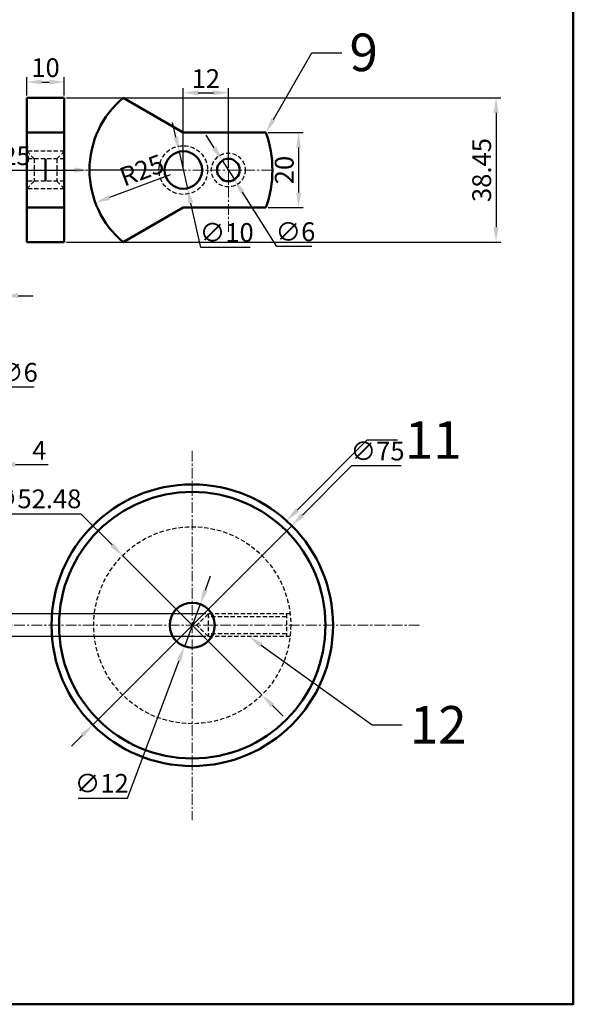
# Model space of a CAD drawing. Units: millimetres. Extents: x 24 to 508, y -182 to 223.
# Tile 5 of 6: x 361 to 508, y -182 to 81. Entities that reach past the tile are written whole.
import ezdxf
from ezdxf import colors
from ezdxf.entities.mleader import LeaderData, LeaderLine
from ezdxf.math import Vec2, Vec3

# ---------------------------------------------------------------- set-up
doc = ezdxf.new("R2010")
doc.units = ezdxf.units.MM
doc.header["$LTSCALE"] = 0.3
doc.linetypes.add('CENTER', pattern=[50.8, 31.75, -6.35, 6.35, -6.35])
doc.linetypes.add('DASHED', pattern=[19.05, 12.7, -6.35])
for name, color, linetype, lineweight in [('M-CNTR', 1, 'CENTER', 18), ('M-DIMS', 2, 'Continuous', 25), ('M-HIDN', 4, 'DASHED', 25), ('M-OUTL', 7, 'Continuous', 50)]:
    doc.layers.add(name, color=color, linetype=linetype, lineweight=lineweight)
doc.styles.get("Standard").update_dxf_attribs({"font": 'arial.ttf'})
doc.dimstyles.new('ISO-25', dxfattribs={"dimtxt": 5, "dimasz": 4, "dimexe": 1.25, "dimexo": 0.625, "dimtad": 1, "dimtoh": 1, "dimdec": 0, "dimtxsty": 'Standard', "dimcen": 2.5, "dimadec": 0, "dimazin": 0, "dimtfac": 1, "dimtdec": 0, "dimtmove": 0, "dimatfit": 3, "dimfxl": 1, "dimarcsym": 0})

# ---------------------------------------------------------------- blocks, each defined once
blk = doc.blocks.new('*D36')
at = {"layer": 'Defpoints', "color": 0, "ltscale": 0.3, "transparency": 16777216}
for p in [(356.48, 7.17), (348.48, -8.39), (356.48, -8.39)]:
    blk.add_point(p, dxfattribs=at)
at = {"layer": 'M-DIMS', "color": 0, "lineweight": -2, "ltscale": 0.3, "transparency": 16777216}
for p, q in [((348.48, -7.76), (348.48, 8.42)), ((356.48, -7.76), (356.48, 8.42)), ((344.48, 7.17), (340.48, 7.17)), ((348.48, 7.17), (356.48, 7.17)), ((360.48, 7.17), (364.48, 7.17))]:
    blk.add_line(p, q, dxfattribs=at)
at = {"layer": 'M-DIMS', "color": 0, "ltscale": 0.3, "transparency": 16777216}
for points in [[(344.48, 7.84), (344.48, 6.51), (348.48, 7.17)], [(360.48, 7.84), (360.48, 6.51), (356.48, 7.17)]]:
    blk.add_solid(points, dxfattribs=at)
at = {"layer": 'M-DIMS', "color": 0, "ltscale": 0.3, "transparency": 16777216, "insert": (352.48, 10.35), "char_height": 5, "attachment_point": 5}
blk.add_mtext('8', dxfattribs=at)
blk = doc.blocks.new('*D38')
at = {"layer": 'Defpoints', "color": 0, "ltscale": 0.3, "transparency": 16777216}
for p in [(347.2, 0.33), (349.76, -5.1)]:
    blk.add_point(p, dxfattribs=at)
at = {"layer": 'M-DIMS', "color": 0, "lineweight": -2, "ltscale": 0.3, "transparency": 16777216}
for p, q in [((345.5, 3.95), (343.8, 7.57)), ((347.2, 0.33), (349.76, -5.1)), ((355.46, -17.21), (351.47, -8.72)), ((364.8, -17.21), (355.46, -17.21))]:
    blk.add_line(p, q, dxfattribs=at)
at = {"layer": 'M-DIMS', "color": 0, "ltscale": 0.3, "transparency": 16777216}
for points in [[(346.1, 4.23), (344.9, 3.66), (347.2, 0.33)], [(352.07, -8.43), (350.86, -9), (349.76, -5.1)]]:
    blk.add_solid(points, dxfattribs=at)
at = {"layer": 'M-DIMS', "color": 0, "ltscale": 0.3, "transparency": 16777216, "insert": (360.45, -13.89), "char_height": 5, "attachment_point": 5}
blk.add_mtext('∅6', dxfattribs=at)
blk = doc.blocks.new('*D39')
at = {"layer": 'Defpoints', "color": 0, "ltscale": 0.3, "transparency": 16777216}
for p in [(372.81, 64.09), (362.81, 59.87), (372.81, 59.87)]:
    blk.add_point(p, dxfattribs=at)
at = {"layer": 'M-DIMS', "color": 0, "lineweight": -2, "ltscale": 0.3, "transparency": 16777216}
for p, q in [((362.81, 60.49), (362.81, 65.34)), ((366.81, 64.09), (368.81, 64.09)), ((372.81, 60.49), (372.81, 65.34))]:
    blk.add_line(p, q, dxfattribs=at)
at = {"layer": 'M-DIMS', "color": 0, "ltscale": 0.3, "transparency": 16777216}
for points in [[(366.81, 64.75), (366.81, 63.42), (362.81, 64.09)], [(368.81, 64.75), (368.81, 63.42), (372.81, 64.09)]]:
    blk.add_solid(points, dxfattribs=at)
at = {"layer": 'M-DIMS', "color": 0, "ltscale": 0.3, "transparency": 16777216, "insert": (367.81, 67.26), "char_height": 5, "attachment_point": 5}
blk.add_mtext('10', dxfattribs=at)
blk = doc.blocks.new('*D40')
at = {"layer": 'Defpoints', "color": 0, "ltscale": 0.3, "transparency": 16777216}
for p in [(404.52, 40.64), (381.09, 31.92)]:
    blk.add_point(p, dxfattribs=at)
at = {"layer": 'M-DIMS', "color": 0, "lineweight": -2, "ltscale": 0.3, "transparency": 16777216}
blk.add_line((400.99, 39.33), (384.84, 33.32), dxfattribs=at)
at = {"layer": 'M-DIMS', "color": 0, "ltscale": 0.3, "transparency": 16777216}
blk.add_solid([(384.6, 33.94), (385.07, 32.69), (381.09, 31.92)], dxfattribs=at)
at = {"layer": 'M-DIMS', "color": 0, "ltscale": 0.3, "transparency": 16777216, "insert": (393.68, 40), "char_height": 5, "attachment_point": 5, "rotation": 20.4111}
blk.add_mtext('R25', dxfattribs=at)
blk = doc.blocks.new('*D41')
at = {"layer": 'Defpoints', "color": 0, "ltscale": 0.3, "transparency": 16777216}
for p in [(416.52, 61.22), (404.52, 40.64), (416.52, 40.64)]:
    blk.add_point(p, dxfattribs=at)
at = {"layer": 'M-DIMS', "color": 0, "lineweight": -2, "ltscale": 0.3, "transparency": 16777216}
for p, q in [((404.52, 41.27), (404.52, 62.47)), ((408.52, 61.22), (412.52, 61.22)), ((416.52, 41.27), (416.52, 62.47))]:
    blk.add_line(p, q, dxfattribs=at)
at = {"layer": 'M-DIMS', "color": 0, "ltscale": 0.3, "transparency": 16777216}
for points in [[(408.52, 61.89), (408.52, 60.56), (404.52, 61.22)], [(412.52, 61.89), (412.52, 60.56), (416.52, 61.22)]]:
    blk.add_solid(points, dxfattribs=at)
at = {"layer": 'M-DIMS', "color": 0, "ltscale": 0.3, "transparency": 16777216, "insert": (410.52, 64.36), "char_height": 5, "attachment_point": 5}
blk.add_mtext('12', dxfattribs=at)
blk = doc.blocks.new('*D42')
at = {"layer": 'Defpoints', "color": 0, "ltscale": 0.3, "transparency": 16777216}
for p in [(426.52, 50.64), (426.52, 30.64), (435.24, 30.64)]:
    blk.add_point(p, dxfattribs=at)
at = {"layer": 'M-DIMS', "color": 0, "lineweight": -2, "ltscale": 0.3, "transparency": 16777216}
for p, q in [((427.14, 50.64), (436.49, 50.64)), ((435.24, 46.64), (435.24, 34.64)), ((427.14, 30.64), (436.49, 30.64))]:
    blk.add_line(p, q, dxfattribs=at)
at = {"layer": 'M-DIMS', "color": 0, "ltscale": 0.3, "transparency": 16777216}
for points in [[(434.58, 46.64), (435.91, 46.64), (435.24, 50.64)], [(434.58, 34.64), (435.91, 34.64), (435.24, 30.64)]]:
    blk.add_solid(points, dxfattribs=at)
at = {"layer": 'M-DIMS', "color": 0, "ltscale": 0.3, "transparency": 16777216, "insert": (432.06, 40.64), "char_height": 5, "attachment_point": 5, "rotation": 90}
blk.add_mtext('20', dxfattribs=at)
blk = doc.blocks.new('*D43')
at = {"layer": 'Defpoints', "color": 0, "ltscale": 0.3, "transparency": 16777216}
for p in [(403.42, 45.52), (405.62, 35.76)]:
    blk.add_point(p, dxfattribs=at)
at = {"layer": 'M-DIMS', "color": 0, "lineweight": -2, "ltscale": 0.3, "transparency": 16777216}
for p, q in [((402.54, 49.42), (401.66, 53.33)), ((403.42, 45.52), (405.62, 35.76)), ((409.16, 20.04), (406.49, 31.86)), ((422.37, 20.04), (409.16, 20.04))]:
    blk.add_line(p, q, dxfattribs=at)
at = {"layer": 'M-DIMS', "color": 0, "ltscale": 0.3, "transparency": 16777216}
for points in [[(403.19, 49.57), (401.89, 49.28), (403.42, 45.52)], [(407.14, 32.01), (405.84, 31.72), (405.62, 35.76)]]:
    blk.add_solid(points, dxfattribs=at)
at = {"layer": 'M-DIMS', "color": 0, "ltscale": 0.3, "transparency": 16777216, "insert": (416.08, 23.36), "char_height": 5, "attachment_point": 5}
blk.add_mtext('∅10', dxfattribs=at)
blk = doc.blocks.new('*D44')
at = {"layer": 'Defpoints', "color": 0, "ltscale": 0.3, "transparency": 16777216}
for p in [(414.91, 43.18), (418.12, 38.11)]:
    blk.add_point(p, dxfattribs=at)
at = {"layer": 'M-DIMS', "color": 0, "lineweight": -2, "ltscale": 0.3, "transparency": 16777216}
for p, q in [((412.78, 46.56), (410.64, 49.94)), ((414.91, 43.18), (418.12, 38.11)), ((429.41, 20.24), (420.26, 34.73)), ((438.75, 20.24), (429.41, 20.24))]:
    blk.add_line(p, q, dxfattribs=at)
at = {"layer": 'M-DIMS', "color": 0, "ltscale": 0.3, "transparency": 16777216}
for points in [[(413.34, 46.92), (412.21, 46.2), (414.91, 43.18)], [(420.82, 35.08), (419.69, 34.37), (418.12, 38.11)]]:
    blk.add_solid(points, dxfattribs=at)
at = {"layer": 'M-DIMS', "color": 0, "ltscale": 0.3, "transparency": 16777216, "insert": (434.39, 23.56), "char_height": 5, "attachment_point": 5}
blk.add_mtext('∅6', dxfattribs=at)
blk = doc.blocks.new('*D53')
at = {"layer": 'Defpoints', "color": 0, "ltscale": 0.3, "transparency": 16777216}
for p in [(409, -74.99), (404.8, -86.23)]:
    blk.add_point(p, dxfattribs=at)
at = {"layer": 'M-DIMS', "color": 0, "lineweight": -2, "ltscale": 0.3, "transparency": 16777216}
for p, q in [((410.4, -71.24), (411.8, -67.49)), ((409, -74.99), (404.8, -86.23)), ((389.69, -126.69), (403.4, -89.97)), ((376.52, -126.69), (389.69, -126.69))]:
    blk.add_line(p, q, dxfattribs=at)
at = {"layer": 'M-DIMS', "color": 0, "ltscale": 0.3, "transparency": 16777216}
for points in [[(409.77, -71.01), (411.02, -71.47), (409, -74.99)], [(402.78, -89.74), (404.03, -90.21), (404.8, -86.23)]]:
    blk.add_solid(points, dxfattribs=at)
at = {"layer": 'M-DIMS', "color": 0, "ltscale": 0.3, "transparency": 16777216, "insert": (382.79, -123.37), "char_height": 5, "attachment_point": 5}
blk.add_mtext('∅12', dxfattribs=at)
blk = doc.blocks.new('*D54')
at = {"layer": 'Defpoints', "color": 0, "ltscale": 0.3, "transparency": 16777216}
for p in [(355.8, -37.78), (351.8, -43.11), (355.8, -43.11)]:
    blk.add_point(p, dxfattribs=at)
at = {"layer": 'M-DIMS', "color": 0, "lineweight": -2, "ltscale": 0.3, "transparency": 16777216}
for p, q in [((351.8, -42.48), (351.8, -36.53)), ((355.8, -42.48), (355.8, -36.53)), ((347.8, -37.78), (343.8, -37.78)), ((351.8, -37.78), (355.8, -37.78)), ((359.8, -37.78), (368.51, -37.78))]:
    blk.add_line(p, q, dxfattribs=at)
at = {"layer": 'M-DIMS', "color": 0, "ltscale": 0.3, "transparency": 16777216}
for points in [[(347.8, -37.11), (347.8, -38.44), (351.8, -37.78)], [(359.8, -37.11), (359.8, -38.44), (355.8, -37.78)]]:
    blk.add_solid(points, dxfattribs=at)
at = {"layer": 'M-DIMS', "color": 0, "ltscale": 0.3, "transparency": 16777216, "insert": (366.15, -34.65), "char_height": 5, "attachment_point": 5}
blk.add_mtext('4', dxfattribs=at)
blk = doc.blocks.new('*D75')
at = {"layer": 'Defpoints', "color": 0, "ltscale": 0.3, "transparency": 16777216}
for p in [(372.81, 59.87), (372.81, 21.42), (487.84, 21.42)]:
    blk.add_point(p, dxfattribs=at)
at = {"layer": 'M-DIMS', "color": 0, "lineweight": -2, "ltscale": 0.3, "transparency": 16777216}
for p, q in [((373.44, 59.87), (489.09, 59.87)), ((487.84, 55.87), (487.84, 25.42)), ((373.44, 21.42), (489.09, 21.42))]:
    blk.add_line(p, q, dxfattribs=at)
at = {"layer": 'M-DIMS', "color": 0, "ltscale": 0.3, "transparency": 16777216}
for points in [[(487.17, 55.87), (488.5, 55.87), (487.84, 59.87)], [(487.17, 25.42), (488.5, 25.42), (487.84, 21.42)]]:
    blk.add_solid(points, dxfattribs=at)
at = {"layer": 'M-DIMS', "color": 0, "ltscale": 0.3, "transparency": 16777216, "insert": (484.66, 40.64), "char_height": 5, "attachment_point": 5, "rotation": 90}
blk.add_mtext('38.45', dxfattribs=at)
blk = doc.blocks.new('*D76')
at = {"layer": 'Defpoints', "color": 0, "ltscale": 0.3, "transparency": 16777216}
for p in [(411.13, -77.61), (56.57, -83.61), (411.13, -83.61)]:
    blk.add_point(p, dxfattribs=at)
at = {"layer": 'M-DIMS', "color": 0, "lineweight": -2, "ltscale": 0.3, "transparency": 16777216}
for p, q in [((56.57, -73.61), (56.57, -69.61)), ((410.51, -77.61), (55.32, -77.61)), ((56.57, -77.61), (56.57, -83.61)), ((410.51, -83.61), (55.32, -83.61)), ((56.57, -87.61), (56.57, -91.61))]:
    blk.add_line(p, q, dxfattribs=at)
at = {"layer": 'M-DIMS', "color": 0, "ltscale": 0.3, "transparency": 16777216}
for points in [[(55.9, -73.61), (57.24, -73.61), (56.57, -77.61)], [(55.9, -87.61), (57.24, -87.61), (56.57, -83.61)]]:
    blk.add_solid(points, dxfattribs=at)
at = {"layer": 'M-DIMS', "color": 0, "ltscale": 0.3, "transparency": 16777216, "insert": (53.39, -80.61), "char_height": 5, "attachment_point": 5, "rotation": 90}
blk.add_mtext('6', dxfattribs=at)
blk = doc.blocks.new('*D83')
at = {"layer": 'Defpoints', "color": 0, "ltscale": 0.3, "transparency": 16777216}
for p in [(379.52, 40.64), (404.52, 40.64)]:
    blk.add_point(p, dxfattribs=at)
at = {"layer": 'M-DIMS', "color": 0, "lineweight": -2, "ltscale": 0.3, "transparency": 16777216}
for p, q in [((351.91, 40.64), (364.52, 40.64)), ((364.52, 40.64), (375.52, 40.64)), ((404.52, 40.64), (379.52, 40.64))]:
    blk.add_line(p, q, dxfattribs=at)
at = {"layer": 'M-DIMS', "color": 0, "ltscale": 0.3, "transparency": 16777216}
blk.add_solid([(375.52, 41.31), (375.52, 39.98), (379.52, 40.64)], dxfattribs=at)
at = {"layer": 'M-DIMS', "color": 0, "ltscale": 0.3, "transparency": 16777216, "insert": (357.9, 43.82), "char_height": 5, "attachment_point": 5}
blk.add_mtext('R25', dxfattribs=at)
blk = doc.blocks.new('*D84')
at = {"layer": 'Defpoints', "color": 0, "ltscale": 0.3, "transparency": 16777216}
for p in [(433.41, -54.09), (380.39, -107.13)]:
    blk.add_point(p, dxfattribs=at)
at = {"layer": 'M-DIMS', "color": 0, "lineweight": -2, "ltscale": 0.3, "transparency": 16777216}
for p, q in [((449.32, -38.17), (436.24, -51.26)), ((462.59, -38.17), (449.32, -38.17)), ((380.39, -107.13), (433.41, -54.09)), ((377.56, -109.96), (374.73, -112.78))]:
    blk.add_line(p, q, dxfattribs=at)
at = {"layer": 'M-DIMS', "color": 0, "ltscale": 0.3, "transparency": 16777216}
for points in [[(435.77, -50.79), (436.71, -51.73), (433.41, -54.09)], [(377.09, -109.48), (378.03, -110.43), (380.39, -107.13)]]:
    blk.add_solid(points, dxfattribs=at)
at = {"layer": 'M-DIMS', "color": 0, "ltscale": 0.3, "transparency": 16777216, "insert": (456.27, -34.86), "char_height": 5, "attachment_point": 5}
blk.add_mtext('∅75', dxfattribs=at)
blk = doc.blocks.new('*D85')
at = {"layer": 'Defpoints', "color": 0, "ltscale": 0.3, "transparency": 16777216}
for p in [(388.35, -62.05), (425.45, -99.17)]:
    blk.add_point(p, dxfattribs=at)
at = {"layer": 'M-DIMS', "color": 0, "lineweight": -2, "ltscale": 0.3, "transparency": 16777216}
for p, q in [((354.27, -50.91), (377.22, -50.91)), ((377.22, -50.91), (385.52, -59.22)), ((425.45, -99.17), (388.35, -62.05)), ((428.28, -101.99), (431.11, -104.82))]:
    blk.add_line(p, q, dxfattribs=at)
at = {"layer": 'M-DIMS', "color": 0, "ltscale": 0.3, "transparency": 16777216}
for points in [[(385.99, -58.75), (385.05, -59.69), (388.35, -62.05)], [(428.75, -101.52), (427.81, -102.47), (425.45, -99.17)]]:
    blk.add_solid(points, dxfattribs=at)
at = {"layer": 'M-DIMS', "color": 0, "ltscale": 0.3, "transparency": 16777216, "insert": (365.43, -47.59), "char_height": 5, "attachment_point": 5}
blk.add_mtext('∅52.48', dxfattribs=at)

msp = doc.modelspace()

# ---------------------------------------------------------------- linework, layer by layer
at = {"layer": 'M-CNTR', "ltscale": 0.3}
for p, q in [((416.5166, 24.1494), (416.5166, 54.5542)), ((428.1856, 40.6427), (347.5151, 40.6427)), ((406.9005, -34.1091), (406.9005, -132.5474)), ((467.488, -80.6068), (308.7003, -80.6068))]:
    msp.add_line(p, q, dxfattribs=at)
at = {"layer": 'M-HIDN', "ltscale": 0.3}
for p, q in [((372.8147, 45.6427), (362.8147, 45.6427)), ((364.8147, 43.6427), (362.8147, 45.6427)), ((370.8147, 43.6427), (372.8147, 45.6427)), ((372.8147, 43.6427), (362.8147, 43.6427)), ((364.8147, 43.6427), (364.8147, 37.6427)), ((370.8147, 43.6427), (370.8147, 37.6427)), ((372.8147, 37.6427), (362.8147, 37.6427)), ((364.8147, 37.6427), (362.8147, 35.6427)), ((370.8147, 37.6427), (372.8147, 35.6427)), ((372.8147, 35.6427), (362.8147, 35.6427)), ((411.1321, -77.6068), (408.1321, -80.6068)), ((432.9701, -77.6068), (411.1321, -77.6068)), ((411.1321, -77.6068), (411.1321, -83.6068)), ((431.9752, -78.3568), (411.1321, -78.3568)), ((431.9752, -77.6068), (431.9752, -83.6068)), ((411.1321, -83.6068), (408.1321, -80.6068)), ((431.9752, -82.8568), (411.1321, -82.8568)), ((432.9701, -83.6068), (411.1321, -83.6068))]:
    msp.add_line(p, q, dxfattribs=at)
for centre, radius in [((404.5166, 40.6427), 6.5), ((416.5166, 40.6427), 4.5), ((406.9005, -80.6068), 26.2417)]:
    msp.add_circle(centre, radius, dxfattribs=at)
at = {"layer": 'M-OUTL', "ltscale": 0.3}
for p, q in [((372.8147, 59.8688), (362.8147, 59.8688)), ((362.8147, 59.8688), (362.8147, 21.4167)), ((372.8147, 40.6427), (372.8147, 59.8688)), ((404.5166, 50.6427), (388.5366, 59.8688)), ((372.8147, 50.6427), (362.8147, 50.6427)), ((416.5166, 50.6427), (404.5166, 50.6427)), ((416.5166, 50.6427), (426.5166, 50.6427)), ((367.8147, 43.6427), (367.8147, 37.6427)), ((372.8147, 21.4167), (372.8147, 40.6427)), ((372.8147, 30.6427), (362.8147, 30.6427)), ((404.5166, 30.6427), (388.5366, 21.4167)), ((416.5166, 30.6427), (404.5166, 30.6427)), ((426.5166, 30.6427), (416.5166, 30.6427)), ((362.8147, 21.4167), (372.8147, 21.4167))]:
    msp.add_line(p, q, dxfattribs=at)
msp.add_lwpolyline([(23.7253, 222.7463), (508.4225, 222.7463), (508.4225, -181.5799), (23.7253, -181.5799)], close=True, dxfattribs=at)
for centre, radius in [((404.5166, 40.6427), 5), ((416.5166, 40.6427), 3), ((406.9005, -80.6068), 37.5), ((406.9005, -80.6068), 35.5), ((406.9005, -80.6068), 6)]:
    msp.add_circle(centre, radius, dxfattribs=at)
for centre, radius, start, end in [((404.5166, 40.6427), 25, 129.732099, 230.267901), ((398.7061, 40.6427), 29.5537, 340.222598, 19.777402)]:
    msp.add_arc(centre, radius, start, end, dxfattribs=at)

# ---------------------------------------------------------------- dimensions: what is measured, and where the dimension line sits
at = {"layer": 'M-DIMS', "ltscale": 0.3}
for base, p1, p2, picture, middle in [((372.8147, 64.0859), (362.8147, 59.8688), (372.8147, 59.8688), '*D39', (367.8147, 67.2638)), ((416.5166, 61.2226), (404.5166, 40.6427), (416.5166, 40.6427), '*D41', (410.5166, 64.3579)), ((356.4824, 7.1732), (348.4824, -8.3853), (356.4824, -8.3853), '*D36', (352.4824, 10.3511)), ((355.8004, -37.7754), (351.8004, -43.1068), (355.8004, -43.1068), '*D54', (366.1546, -34.6504))]:
    dim = msp.add_linear_dim(base=base, p1=p1, p2=p2, dimstyle='ISO-25', override={"dimclrd": 0, "dimclre": 0, "dimclrt": 0}, dxfattribs=at)
    dim.commit()
    dim.dimension.update_dxf_attribs({"geometry": picture, "text_midpoint": middle})
for base, p1, p2, override, picture, middle in [((487.838, 21.4167), (372.8147, 59.8688), (372.8147, 21.4167), {"dimdec": 2, "dimlfac": 1, "dimrnd": 0, "dimzin": 0, "dimdsep": 46, "dimlunit": 2}, '*D75', (484.6585, 40.6427)), ((435.2422, 30.6427), (426.5166, 50.6427), (426.5166, 30.6427), {"dimclrd": 0, "dimclre": 0, "dimclrt": 0}, '*D42', (432.0643, 40.6427)), ((56.5704, -83.6068), (411.1321, -77.6068), (411.1321, -83.6068), {"dimdec": 0, "dimlfac": 1, "dimrnd": 0, "dimzin": 0, "dimdsep": 46, "dimlunit": 2}, '*D76', (53.3925, -80.6068))]:
    dim = msp.add_linear_dim(base=base, p1=p1, p2=p2, angle=90, dimstyle='ISO-25', override=override, dxfattribs=at)
    dim.commit()
    dim.dimension.update_dxf_attribs({"geometry": picture, "text_midpoint": middle})
for p1, p2, override, picture, middle in [((403.4179, 45.5205), (405.6153, 35.765), {"dimclrd": 0, "dimclre": 0, "dimclrt": 0}, '*D43', (416.0754, 20.0378)), ((414.9137, 43.1786), (418.1195, 38.1069), {"dimclrd": 0, "dimclre": 0, "dimclrt": 0}, '*D44', (434.3937, 20.2422)), ((380.3876, -107.1269), (433.4133, -54.0867), {"dimdec": 0, "dimlfac": 1, "dimrnd": 0, "dimzin": 0, "dimdsep": 46, "dimlunit": 2}, '*D84', (456.266, -38.1746)), ((425.453, -99.1656), (388.348, -62.048), {"dimdec": 2, "dimlfac": 1, "dimrnd": 0, "dimzin": 0, "dimdsep": 46, "dimlunit": 2}, '*D85', (365.4301, -50.9127)), ((408.9994, -74.9859), (404.8016, -86.2277), {"dimclrd": 0, "dimclre": 0, "dimclrt": 0}, '*D53', (382.7926, -126.688))]:
    dim = msp.add_diameter_dim_2p(p1=p1, p2=p2, dimstyle='ISO-25', override=override, dxfattribs=at)
    dim.commit()
    dim.dimension.update_dxf_attribs({"geometry": picture, "text_midpoint": middle, "dimtype": 163})
for mpoint, override, picture, middle in [((379.5166, 40.643), {"dimdec": 0, "dimlfac": 1, "dimrnd": 0, "dimzin": 0, "dimdsep": 46, "dimlunit": 2}, '*D83', (364.5166, 40.6432)), ((381.0862, 31.9239), {"dimclrd": 0, "dimclre": 0, "dimclrt": 0}, '*D40', (394.786, 37.0218))]:
    dim = msp.add_radius_dim(center=(404.5166, 40.6427), mpoint=mpoint, dimstyle='ISO-25', override=override, dxfattribs=at)
    dim.commit()
    dim.dimension.update_dxf_attribs({"geometry": picture, "text_midpoint": middle, "dimtype": 164})
dim = msp.add_diameter_dim_2p(p1=(347.2042, 0.3287), p2=(349.7607, -5.0994), dimstyle='ISO-25', override={"dimclrd": 0, "dimclre": 0, "dimclrt": 0}, dxfattribs=at)
dim.commit()
dim.dimension.update_dxf_attribs({"geometry": '*D38', "text_midpoint": (360.446, -13.8913)})

# ---------------------------------------------------------------- leaders
ml = msp.add_multileader_mtext('Standard', dxfattribs=at)
ml.set_content('9', color=256)
ml.set_leader_properties()
ml.build(insert=Vec2(0, 0))
ctx = ml.context
ctx.base_point, ctx.char_height, ctx.plane_origin = Vec3(446.7899, 71.9008), 10, Vec3(426.5166, 50.6427)
notes = []
notes.append((ctx, [(0, (1, 1, 0), (438.7899, 71.9008), (1, 0), 8, [(0, [(426.5166, 50.6427)], 0, [])])]))
ctx.mtext.insert, ctx.mtext.flow_direction = Vec3(448.7899, 76.986), 5
ml = msp.add_multileader_mtext('Standard', dxfattribs=at)
ml.set_content('11', color=256)
ml.set_leader_properties()
ml.build(insert=Vec2(0, 0))
ctx = ml.context
ctx.base_point, ctx.char_height, ctx.plane_origin = Vec3(461.5416, -31.2626), 10, Vec3(432.031, -52.7732)
notes.append((ctx, [(0, (1, 1, 0), (453.5416, -31.2626), (1, 0), 8, [(0, [(432.031, -52.7732)], 0, [])])]))
ctx.mtext.insert, ctx.mtext.flow_direction = Vec3(463.5416, -26.2626), 5
ml = msp.add_multileader_mtext('Standard', dxfattribs=at)
ml.set_content('12', color=256)
ml.set_leader_properties()
ml.build(insert=Vec2(0, 0))
ctx = ml.context
ctx.base_point, ctx.char_height, ctx.plane_origin = Vec3(462.8649, -107.1329), 10, Vec3(422.0511, -83.6068)
notes.append((ctx, [(0, (1, 1, 0), (454.8649, -107.1329), (1, 0), 8, [(0, [(422.0511, -83.6068)], 0, [])])]))
ctx.mtext.insert, ctx.mtext.flow_direction = Vec3(464.8649, -102.1329), 5
for ctx, leaders in notes:
    for number, flags, end, landing, length, lines in leaders:
        leader = LeaderData()
        leader.index, (leader.has_last_leader_line, leader.has_dogleg_vector, leader.attachment_direction) = number, flags
        leader.last_leader_point, leader.dogleg_vector, leader.dogleg_length = Vec3(end), Vec3(landing), length
        for number, points, colour, breaks in lines:
            line = LeaderLine()
            line.index, line.vertices, line.color, line.breaks = number, Vec3.list(points), colors.encode_raw_color(colour), breaks
            leader.lines.append(line)
        ctx.leaders.append(leader)

doc.saveas('drawing.dxf')
